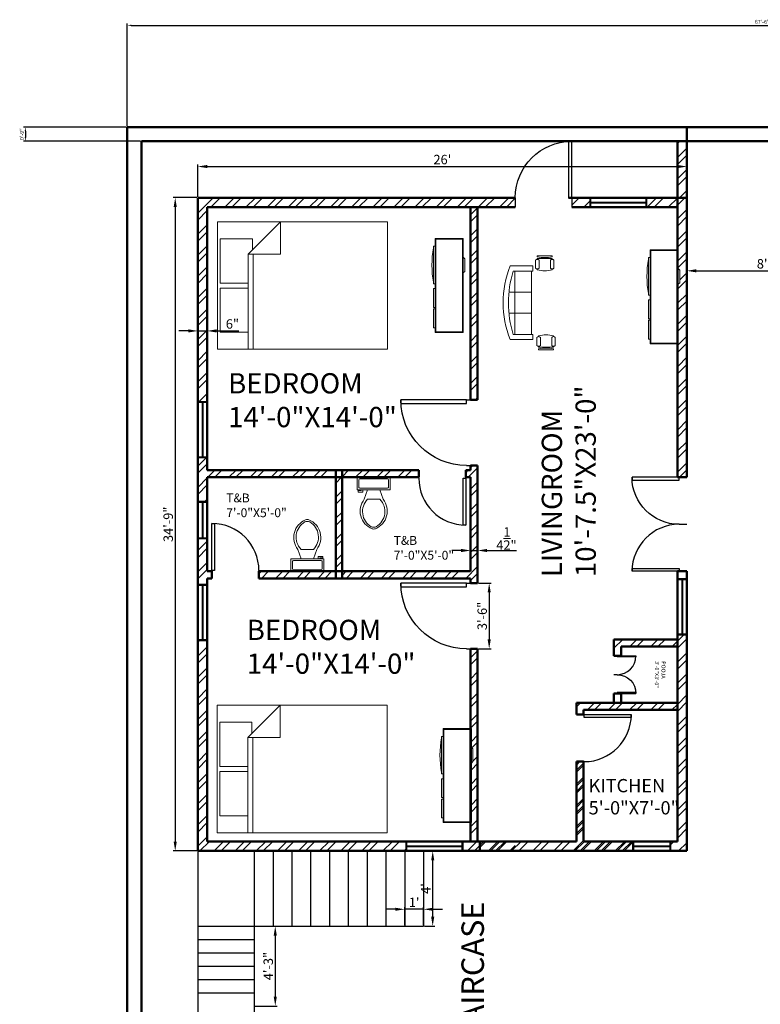
# Model space of a CAD drawing. Units: inches. Extents: x -12550 to 6516, y 1273 to 18700.
# Tile 10 of 19: x 3066 to 3538, y 1958 to 2587. Entities that reach past the tile are written whole.
import ezdxf

# ---------------------------------------------------------------- set-up
doc = ezdxf.new("R2010")
doc.units = ezdxf.units.IN
for name, color, linetype, lineweight in [('A-ANNO-DIMS', 2, 'Continuous', 18), ('A-AREA-IDEN', 1, 'Continuous', 18), ('A-DOOR', 5, 'Continuous', 25), ('A-FLOR-STRS', 6, 'Continuous', 25), ('A-FURN', 8, 'Continuous', 18), ('A-GLAZ', 3, 'Continuous', 25), ('A-WALL', 7, 'Continuous', 50), ('A-WALL-PATT', 8, 'Continuous', 13)]:
    doc.layers.add(name, color=color, linetype=linetype, lineweight=lineweight)
doc.styles.get("Standard").update_dxf_attribs({"font": 'arial.ttf'})
doc.dimstyles.new('ISO-25', dxfattribs={"dimtxt": 2.5, "dimasz": 2.5, "dimexe": 1.25, "dimexo": 0.625, "dimtad": 1, "dimlunit": 4, "dimtxsty": 'Standard', "dimcen": 2.5, "dimadec": 0, "dimazin": 0, "dimtfac": 1, "dimtmove": 0, "dimatfit": 3, "dimfxl": 1, "dimarcsym": 0})
pattern_1 = [(45, (1161.5385, 0), (-6.735192, 6.735192), []), (45, (1166.029, 0), (-6.735192, 6.735192), [])]
pattern_2 = [(45, (1161.5385, 567), (-6.735192, 6.735192), []), (45, (1166.029, 567), (-6.735192, 6.735192), [])]

# ---------------------------------------------------------------- blocks, each defined once
blk = doc.blocks.new('*U2')
for p, q in [((0, 0), (0, -5)), ((30, 0), (30, -5))]:
    blk.add_line(p, q)
blk.add_lwpolyline([(0, 0), (0, 30), (1.75, 30), (1.75, 0)], close=True)
blk.add_arc((0, 0), 30, 0, 90)
blk = doc.blocks.new('Bed - Queen')
for p, q in [((0, -80.00003), (0, 0)), ((0, 0), (59.99999, 0)), ((59.99999, 0), (59.99999, -80.00003)), ((7.99999, -1.2), (28.79998, -1.2)), ((7.99999, -14.4), (7.99999, -1.2)), ((28.79998, -1.2), (28.79998, -14.4)), ((31.19999, -1.2), (51.99999, -1.2)), ((31.19999, -14.4), (31.19999, -1.2)), ((51.99999, -1.2), (51.99999, -16.4)), ((0, -14.4), (44.8, -14.4)), ((44.8, -16.8), (0, -16.8)), ((59.99999, -29.6), (44.8, -14.4)), ((44.8, -14.4), (44.8, -29.6)), ((51.99999, -16.4), (46.79936, -16.4)), ((44.8, -29.6), (59.99999, -29.6)), ((59.99999, -80.00003), (0, -80.00003))]:
    blk.add_line(p, q)
blk = doc.blocks.new('Toilet - top')
for p, q in [((9.5, -6), (9.5, -2)), ((-10, -8.5), (-8, -8.5)), ((-10, -9.5), (-10, -8.5)), ((-7, -9.5), (-10, -9.5)), ((-8, -8.5), (-8, -8)), ((-7, -8), (-7, -9.5)), ((-4, -8), (-6, -14)), ((4, -8), (6, -14)), ((4, -14), (-4, -14))]:
    blk.add_line(p, q)
blk.add_lwpolyline([(10.5, -8), (10.5, 0), (-10.5, 0), (-10.5, -8)], close=True)
for points in [[(-9.5, -2), (-9.5, -6)], [(8.5, -1), (-8.5, -1)], [(-8.5, -7), (8.5, -7)]]:
    blk.add_lwpolyline(points)
for centre, radius, start, end in [((-8.62, -1.88), 0.884, 81.8699, 188.1301), ((-8.62, -6.12), 0.884, 171.8699, 278.1301), ((8.62, -1.88), 0.884, 351.8699, 98.1301), ((8.62, -6.12), 0.884, 261.8699, 8.1301), ((3.52, -21.58), 12.17, 141.46911, 247.97143), ((4.2, -21.82), 11.33, 136.36773, 238.94682), ((-3.52, -21.58), 12.17, 292.02843, 38.53071), ((-4.2, -21.82), 11.33, 301.05301, 43.63209), ((0, -27.88), 4, 245.73182, 294.26817), ((0, -29), 4, 254.86053, 285.13947)]:
    blk.add_arc(centre, radius, start, end)
blk = doc.blocks.new('Entertainment Center')
for p, q in [((-4, 0), (-5, -1)), ((4, 0), (-4, 0)), ((5, -1), (4, 0)), ((-17, -19), (-17, -1)), ((-17, -1), (43, -1)), ((-16.5, -18.5), (-16.5, -1.5)), ((-16.5, -1.5), (42.5, -1.5)), ((42.5, -1.5), (42.5, -18.5)), ((43, -1), (43, -19)), ((42.5, -18.5), (-16.5, -18.5)), ((43, -19), (-17, -19)), ((-12, -20), (-12, -19)), ((12, -20), (-12, -20)), ((12, -19), (12, -20)), ((15, -20), (15, -19)), ((27, -20), (15, -20)), ((27, -19), (27, -20)), ((28, -20), (28, -19)), ((40, -20), (28, -20)), ((40, -19), (40, -20))]:
    blk.add_line(p, q)
blk.add_arc((0, 40), 61, 259.6111, 280.3889)
blk = doc.blocks.new('Sofa - Roundback 7 ft.')
for p, q in [((-12.00002, -32.4421), (-12.00003, -6.5971)), ((11.99997, -32.4421), (11.99998, -6.5971)), ((-36.000027, -34), (-36.000027, -11.4696)), ((-35.999844, -13.3819), (35.9998, -13.3819)), ((35.99998, -34), (35.99998, -11.4696)), ((-36.000027, -32.4421), (35.99998, -32.4421))]:
    blk.add_line(p, q)
for points in [[(-36.000027, -34), (-42.000027, -34), (-42.000027, -8)], [(41.99998, -8), (41.99998, -34), (35.99998, -34)]]:
    blk.add_lwpolyline(points)
for centre, radius, start, end in [((0, -114.25), 114.25, 68.43141, 111.5686), ((-0.00001, -127.1968), 121.1968, 72.72033, 107.2797)]:
    blk.add_arc(centre, radius, start, end)
blk = doc.blocks.new('Chair - Desk')
for p, q in [((-8.5, 0), (-8.5, -1)), ((-8.5, 0), (8.5, 0)), ((8.5, 0), (8.5, -1)), ((-10.5, -5), (-10.5, -14)), ((-8.5, -3), (-8.5, -4)), ((-8.5, -3), (8.5, -3)), ((-6.5, -14), (-6.5, -5)), ((-2, -3), (-2, -1.9355)), ((2, -1.9576), (2, -3)), ((6.5, -5), (6.5, -14)), ((8.5, -3), (8.5, -4)), ((10.5, -14), (10.5, -5)), ((-8.5, -15), (-8.5, -16)), ((8.5, -15), (8.5, -16))]:
    blk.add_line(p, q)
for centre, radius, start, end in [((-8.5, -6.5), 2.5, 36.8699, 143.1301), ((0, 34.625), 36.625, 256.5803, 283.4197), ((8.5, -6.5), 2.5, 36.8699, 143.1301), ((-8.5, -12.5), 2.5, 216.8699, 323.1301), ((0, 19.625), 36.625, 256.5803, 283.4197), ((8.5, -12.5), 2.5, 216.8699, 323.1301)]:
    blk.add_arc(centre, radius, start, end)
blk = doc.blocks.new('*D25')
at = {"layer": 'A-ANNO-DIMS', "color": 0, "lineweight": -2, "transparency": 16777216}
for p, q in [((3179.23, 2388.03), (3179.23, 2389.43)), ((3185.23, 2388.03), (3185.23, 2389.43)), ((3173.23, 2388.18), (3167.23, 2388.18)), ((3179.23, 2388.18), (3185.23, 2388.18)), ((3191.23, 2388.18), (3205.41, 2388.18))]:
    blk.add_line(p, q, dxfattribs=at)
at = {"layer": 'A-ANNO-DIMS', "color": 0, "transparency": 16777216}
for points in [[(3173.23, 2389.18), (3173.23, 2387.18), (3179.23, 2388.18)], [(3191.23, 2389.18), (3191.23, 2387.18), (3185.23, 2388.18)]]:
    blk.add_solid(points, dxfattribs=at)
at = {"layer": 'Defpoints', "color": 0, "transparency": 16777216}
for p in [(3179.23, 2387.4), (3185.23, 2388.18), (3185.23, 2387.4)]:
    blk.add_point(p, dxfattribs=at)
at = {"layer": 'A-ANNO-DIMS', "color": 0, "transparency": 16777216, "insert": (3201.32, 2391.87), "char_height": 6, "attachment_point": 5}
blk.add_mtext('6"', dxfattribs=at)
blk = doc.blocks.new('*D26')
at = {"layer": 'A-ANNO-DIMS', "color": 0, "lineweight": -2, "transparency": 16777216}
for p, q in [((3353.23, 2251.78), (3353.23, 2246.78)), ((3357.73, 2251.78), (3357.73, 2246.78)), ((3347.23, 2248.03), (3341.23, 2248.03)), ((3353.23, 2248.03), (3357.73, 2248.03)), ((3363.73, 2248.03), (3382.49, 2248.03))]:
    blk.add_line(p, q, dxfattribs=at)
at = {"layer": 'A-ANNO-DIMS', "color": 0, "transparency": 16777216}
for points in [[(3347.23, 2249.03), (3347.23, 2247.03), (3353.23, 2248.03)], [(3363.73, 2249.03), (3363.73, 2247.03), (3357.73, 2248.03)]]:
    blk.add_solid(points, dxfattribs=at)
at = {"layer": 'Defpoints', "color": 0, "transparency": 16777216}
for p in [(3353.23, 2252.41), (3357.73, 2252.41), (3357.73, 2248.03)]:
    blk.add_point(p, dxfattribs=at)
at = {"layer": 'A-ANNO-DIMS', "color": 0, "transparency": 16777216, "insert": (3376.11, 2255.68), "char_height": 6, "attachment_point": 5}
blk.add_mtext('4{\\H1x;\\S1/2;}"', dxfattribs=at)
blk = doc.blocks.new('*D33')
at = {"layer": 'A-ANNO-DIMS', "color": 0, "lineweight": -2, "transparency": 16777216}
for p, q in [((3358.35, 2227.25), (3366.36, 2227.25)), ((3365.11, 2221.25), (3365.11, 2191.25)), ((3358.35, 2185.25), (3366.36, 2185.25))]:
    blk.add_line(p, q, dxfattribs=at)
at = {"layer": 'A-ANNO-DIMS', "color": 0, "transparency": 16777216}
for points in [[(3364.11, 2221.25), (3366.11, 2221.25), (3365.11, 2227.25)], [(3364.11, 2191.25), (3366.11, 2191.25), (3365.11, 2185.25)]]:
    blk.add_solid(points, dxfattribs=at)
at = {"layer": 'Defpoints', "color": 0, "transparency": 16777216}
for p in [(3357.73, 2227.25), (3357.73, 2185.25), (3365.11, 2185.25)]:
    blk.add_point(p, dxfattribs=at)
at = {"layer": 'A-ANNO-DIMS', "color": 0, "transparency": 16777216, "insert": (3361.42, 2206.25), "char_height": 6, "attachment_point": 5, "rotation": 90}
blk.add_mtext('3\'-6"', dxfattribs=at)
blk = doc.blocks.new('*D34')
at = {"layer": 'A-ANNO-DIMS', "color": 0, "lineweight": -2, "transparency": 16777216}
for p, q in [((3323.85, 2056.25), (3330.33, 2056.25)), ((3329.08, 2014.25), (3329.08, 2050.25)), ((3323.85, 2008.25), (3330.33, 2008.25))]:
    blk.add_line(p, q, dxfattribs=at)
at = {"layer": 'A-ANNO-DIMS', "color": 0, "transparency": 16777216}
for points in [[(3328.08, 2050.25), (3330.08, 2050.25), (3329.08, 2056.25)], [(3328.08, 2014.25), (3330.08, 2014.25), (3329.08, 2008.25)]]:
    blk.add_solid(points, dxfattribs=at)
at = {"layer": 'Defpoints', "color": 0, "transparency": 16777216}
for p in [(3323.23, 2056.25), (3329.08, 2056.25), (3323.23, 2008.25)]:
    blk.add_point(p, dxfattribs=at)
at = {"layer": 'A-ANNO-DIMS', "color": 0, "transparency": 16777216, "insert": (3325.46, 2032.25), "char_height": 6, "attachment_point": 5, "rotation": 90}
blk.add_mtext("4'", dxfattribs=at)
blk = doc.blocks.new('*D35')
at = {"layer": 'A-ANNO-DIMS', "color": 0, "lineweight": -2, "transparency": 16777216}
for p, q in [((3305.23, 2019.01), (3299.23, 2019.01)), ((3311.23, 2008.87), (3311.23, 2020.26)), ((3323.23, 2019.01), (3311.23, 2019.01)), ((3323.23, 2008.87), (3323.23, 2020.26)), ((3329.23, 2019.01), (3335.23, 2019.01))]:
    blk.add_line(p, q, dxfattribs=at)
at = {"layer": 'A-ANNO-DIMS', "color": 0, "transparency": 16777216}
for points in [[(3305.23, 2020.01), (3305.23, 2018.01), (3311.23, 2019.01)], [(3329.23, 2020.01), (3329.23, 2018.01), (3323.23, 2019.01)]]:
    blk.add_solid(points, dxfattribs=at)
at = {"layer": 'Defpoints', "color": 0, "transparency": 16777216}
for p in [(3311.23, 2019.01), (3311.23, 2008.25), (3323.23, 2008.25)]:
    blk.add_point(p, dxfattribs=at)
at = {"layer": 'A-ANNO-DIMS', "color": 0, "transparency": 16777216, "insert": (3317.23, 2022.65), "char_height": 6, "attachment_point": 5}
blk.add_mtext("1'", dxfattribs=at)
blk = doc.blocks.new('*D36')
at = {"layer": 'A-ANNO-DIMS', "color": 0, "lineweight": -2, "transparency": 16777216}
for p, q in [((3215.85, 2008.25), (3229.9, 2008.25)), ((3228.65, 2002.25), (3228.65, 1963.25)), ((3215.85, 1957.25), (3229.9, 1957.25))]:
    blk.add_line(p, q, dxfattribs=at)
at = {"layer": 'A-ANNO-DIMS', "color": 0, "transparency": 16777216}
for points in [[(3227.65, 2002.25), (3229.65, 2002.25), (3228.65, 2008.25)], [(3227.65, 1963.25), (3229.65, 1963.25), (3228.65, 1957.25)]]:
    blk.add_solid(points, dxfattribs=at)
at = {"layer": 'Defpoints', "color": 0, "transparency": 16777216}
for p in [(3215.23, 2008.25), (3215.23, 1957.25), (3228.65, 1957.25)]:
    blk.add_point(p, dxfattribs=at)
at = {"layer": 'A-ANNO-DIMS', "color": 0, "transparency": 16777216, "insert": (3224.96, 1982.75), "char_height": 6, "attachment_point": 5, "rotation": 90}
blk.add_mtext('4\'-3"', dxfattribs=at)
blk = doc.blocks.new('*D29')
at = {"layer": 'A-ANNO-DIMS', "color": 0, "lineweight": -2, "transparency": 16777216}
for p, q in [((3178.6, 2473.25), (3163.57, 2473.25)), ((3164.82, 2467.25), (3164.82, 2062.25)), ((3178.6, 2056.25), (3163.57, 2056.25))]:
    blk.add_line(p, q, dxfattribs=at)
at = {"layer": 'A-ANNO-DIMS', "color": 0, "transparency": 16777216}
for points in [[(3163.82, 2467.25), (3165.82, 2467.25), (3164.82, 2473.25)], [(3163.82, 2062.25), (3165.82, 2062.25), (3164.82, 2056.25)]]:
    blk.add_solid(points, dxfattribs=at)
at = {"layer": 'Defpoints', "color": 0, "transparency": 16777216}
for p in [(3179.23, 2473.25), (3164.82, 2056.25), (3179.23, 2056.25)]:
    blk.add_point(p, dxfattribs=at)
at = {"layer": 'A-ANNO-DIMS', "color": 0, "transparency": 16777216, "insert": (3161.13, 2264.75), "char_height": 6, "attachment_point": 5, "rotation": 90}
blk.add_mtext('34\'-9"', dxfattribs=at)
blk = doc.blocks.new('*D32')
at = {"layer": 'A-ANNO-DIMS', "color": 0, "lineweight": -2, "transparency": 16777216}
for p, q in [((3179.23, 2473.87), (3179.23, 2494.36)), ((3185.23, 2493.11), (3485.23, 2493.11)), ((3491.23, 2473.87), (3491.23, 2494.36))]:
    blk.add_line(p, q, dxfattribs=at)
at = {"layer": 'A-ANNO-DIMS', "color": 0, "transparency": 16777216}
for points in [[(3185.23, 2494.11), (3185.23, 2492.11), (3179.23, 2493.11)], [(3485.23, 2494.11), (3485.23, 2492.11), (3491.23, 2493.11)]]:
    blk.add_solid(points, dxfattribs=at)
at = {"layer": 'Defpoints', "color": 0, "transparency": 16777216}
for p in [(3491.23, 2493.11), (3179.23, 2473.25), (3491.23, 2473.25)]:
    blk.add_point(p, dxfattribs=at)
at = {"layer": 'A-ANNO-DIMS', "color": 0, "transparency": 16777216, "insert": (3335.23, 2496.8), "char_height": 6, "attachment_point": 5}
blk.add_mtext("26'", dxfattribs=at)
blk = doc.blocks.new('*D27')
at = {"layer": 'A-ANNO-DIMS', "color": 0, "lineweight": -2, "transparency": 16777216}
for p, q in [((3491.23, 2407.12), (3491.23, 2427.81)), ((3497.23, 2426.56), (3581.23, 2426.56)), ((3587.23, 2407.12), (3587.23, 2427.81))]:
    blk.add_line(p, q, dxfattribs=at)
at = {"layer": 'A-ANNO-DIMS', "color": 0, "transparency": 16777216}
for points in [[(3497.23, 2427.56), (3497.23, 2425.56), (3491.23, 2426.56)], [(3581.23, 2427.56), (3581.23, 2425.56), (3587.23, 2426.56)]]:
    blk.add_solid(points, dxfattribs=at)
at = {"layer": 'Defpoints', "color": 0, "transparency": 16777216}
for p in [(3587.23, 2426.56), (3491.23, 2406.5), (3587.23, 2406.5)]:
    blk.add_point(p, dxfattribs=at)
at = {"layer": 'A-ANNO-DIMS', "color": 0, "transparency": 16777216, "insert": (3539.23, 2430.25), "char_height": 6, "attachment_point": 5}
blk.add_mtext("8'", dxfattribs=at)
blk = doc.blocks.new('WIN-3FT')
for p, q in [((0, 0), (0, 6)), ((0, 6), (36.02, 6)), ((36.02, 0), (0, 0)), ((0.5, 0), (0.5, 6)), ((35.52, 3.2), (0.5, 3.2)), ((35.52, 2.8), (0.5, 2.8)), ((35.52, 6), (35.52, 0)), ((36.02, 6), (36.02, 0))]:
    blk.add_line(p, q)
blk = doc.blocks.new('WIN-2FT')
for p, q in [((0, 0), (0, 24.02)), ((0, 24.02), (6, 24.02)), ((0, 23.52), (6, 23.52)), ((2.8, 0.5), (2.8, 23.52)), ((3.2, 0.5), (3.2, 23.52)), ((6, 24.02), (6, 0)), ((6, 0.5), (0, 0.5)), ((6, 0), (0, 0))]:
    blk.add_line(p, q)
blk = doc.blocks.new('*D103')
at = {"layer": 'A-ANNO-DIMS', "color": 0, "lineweight": -2, "transparency": 16777216}
for p, q in [((3134.23, 2518.87), (3134.23, 2584.5)), ((3136.73, 2583.25), (3941.73, 2583.25)), ((3944.23, 2518.87), (3944.23, 2584.5))]:
    blk.add_line(p, q, dxfattribs=at)
at = {"layer": 'A-ANNO-DIMS', "color": 0, "transparency": 16777216}
for points in [[(3136.73, 2583.66), (3136.73, 2582.83), (3134.23, 2583.25)], [(3941.73, 2583.66), (3941.73, 2582.83), (3944.23, 2583.25)]]:
    blk.add_solid(points, dxfattribs=at)
at = {"layer": 'Defpoints', "color": 0, "transparency": 16777216}
for p in [(3944.23, 2583.25), (3134.23, 2518.25), (3944.23, 2518.25)]:
    blk.add_point(p, dxfattribs=at)
at = {"layer": 'A-ANNO-DIMS', "color": 0, "transparency": 16777216, "insert": (3539.23, 2585.15), "char_height": 2.5, "attachment_point": 5}
blk.add_mtext('67\'-6"', dxfattribs=at)
blk = doc.blocks.new('*D111')
at = {"layer": 'A-ANNO-DIMS', "color": 0, "lineweight": -2, "transparency": 16777216}
for p, q in [((3133.6, 2518.25), (3067.98, 2518.25)), ((3069.23, 2515.75), (3069.23, 2511.75)), ((3142.6, 2509.25), (3067.98, 2509.25))]:
    blk.add_line(p, q, dxfattribs=at)
at = {"layer": 'A-ANNO-DIMS', "color": 0, "transparency": 16777216}
for points in [[(3068.81, 2515.75), (3069.64, 2515.75), (3069.23, 2518.25)], [(3068.81, 2511.75), (3069.64, 2511.75), (3069.23, 2509.25)]]:
    blk.add_solid(points, dxfattribs=at)
at = {"layer": 'Defpoints', "color": 0, "transparency": 16777216}
for p in [(3134.23, 2518.25), (3069.23, 2509.25), (3143.23, 2509.25)]:
    blk.add_point(p, dxfattribs=at)
at = {"layer": 'A-ANNO-DIMS', "color": 0, "transparency": 16777216, "insert": (3067.33, 2513.75), "char_height": 2.5, "attachment_point": 5, "rotation": 90}
blk.add_mtext('0\'-9"', dxfattribs=at)

msp = doc.modelspace()

# ---------------------------------------------------------------- hatches: boundary and pattern name
at = {"layer": 'A-WALL-PATT'}
h = msp.add_hatch(dxfattribs=at)
h.set_pattern_fill('ANSI32', color=256)
h.set_pattern_definition(pattern_1)
h.paths.add_polyline_path([(3491.227, 2509.247), (3485.227, 2509.247), (3485.227, 2473.247), (3491.227, 2473.247)])
h = msp.add_hatch(dxfattribs=at)
h.set_pattern_fill('ANSI32', color=256)
h.set_pattern_definition(pattern_2)
h.paths.add_polyline_path([(3185.227, 2467.247), (3359.227, 2467.247), (3359.227, 2473.247), (3179.227, 2473.247), (3179.227, 2343.138), (3185.227, 2343.138)])
h = msp.add_hatch(dxfattribs=at)
h.set_pattern_fill('ANSI32', color=256)
h.set_pattern_definition(pattern_2)
h.paths.add_polyline_path([(3417.727, 2473.247), (3417.727, 2467.247), (3429.479, 2467.247), (3429.479, 2473.247)])
h.paths.add_polyline_path([(3381.727, 2467.247), (3381.727, 2473.247), (3359.227, 2473.247), (3359.227, 2467.247)])
h = msp.add_hatch(dxfattribs=at)
h.set_pattern_fill('ANSI32', color=256)
h.set_pattern_definition(pattern_2)
h.paths.add_polyline_path([(3491.227, 2473.247), (3465.496, 2473.247), (3465.496, 2467.247), (3485.227, 2467.247), (3485.227, 2439.972), (3485.727, 2439.972), (3485.727, 2427.972), (3486.727, 2426.972), (3486.727, 2418.972), (3485.727, 2417.972), (3485.727, 2379.972), (3485.227, 2294.747), (3486.227, 2294.747), (3491.227, 2294.747)])
h = msp.add_hatch(dxfattribs=at)
h.set_pattern_fill('ANSI32', color=256)
h.set_pattern_definition(pattern_2)
h.paths.add_polyline_path([(3357.727, 2467.247), (3353.227, 2467.247), (3353.227, 2344.247), (3357.727, 2344.247)], flags=17)
h = msp.add_hatch(dxfattribs=at)
h.set_pattern_fill('ANSI32', color=256)
h.set_pattern_definition(pattern_2)
h.paths.add_polyline_path([(3267.227, 2299.247), (3185.227, 2299.247), (3185.227, 2307.121), (3179.227, 2307.121), (3179.227, 2279.466), (3185.227, 2279.466), (3185.227, 2294.747), (3267.227, 2294.747)])
h = msp.add_hatch(dxfattribs=at)
h.set_pattern_fill('ANSI32', color=256)
h.set_pattern_definition(pattern_2)
h.paths.add_polyline_path([(3357.727, 2302.247), (3353.227, 2302.247), (3353.227, 2299.247), (3350.227, 2299.247), (3350.227, 2294.747), (3353.227, 2294.747), (3353.227, 2234.747), (3271.227, 2234.747), (3271.227, 2230.247), (3353.227, 2230.247), (3353.227, 2227.247), (3357.727, 2227.247)])
h = msp.add_hatch(dxfattribs=at)
h.set_pattern_fill('ANSI32', color=256)
h.set_pattern_definition(pattern_2)
h.paths.add_polyline_path([(3271.227, 2294.747), (3267.227, 2294.747), (3267.227, 2234.747), (3271.227, 2234.747)])
h = msp.add_hatch(dxfattribs=at)
h.set_pattern_fill('ANSI32', color=256)
h.set_pattern_definition(pattern_2)
h.paths.add_polyline_path([(3320.227, 2299.247), (3271.227, 2299.247), (3271.227, 2294.747), (3320.227, 2294.747)], flags=17)
h = msp.add_hatch(dxfattribs=at)
h.set_pattern_fill('ANSI32', color=256)
h.set_pattern_definition(pattern_2)
h.paths.add_polyline_path([(3185.227, 2255.449), (3179.227, 2255.449), (3179.227, 2226.453), (3185.227, 2226.453), (3185.227, 2230.247), (3188.227, 2230.247), (3188.227, 2234.747), (3185.227, 2234.747)])
h = msp.add_hatch(dxfattribs=at)
h.set_pattern_fill('ANSI32', color=256)
h.set_pattern_definition(pattern_2)
h.paths.add_polyline_path([(3267.227, 2234.747), (3218.227, 2234.747), (3218.227, 2230.247), (3267.227, 2230.247)])
h = msp.add_hatch(dxfattribs=at)
h.set_pattern_fill('ANSI32', color=256)
h.set_pattern_definition(pattern_2)
h.paths.add_polyline_path([(3491.227, 2194.032), (3485.227, 2194.032), (3485.227, 2062.247), (3480.833, 2062.247), (3480.833, 2056.247), (3491.227, 2056.247)])
h = msp.add_hatch(dxfattribs=at)
h.set_pattern_fill('ANSI32', color=256)
h.set_pattern_definition(pattern_2)
h.paths.add_polyline_path([(3185.227, 2190.435), (3179.227, 2190.435), (3179.227, 2056.247), (3312.178, 2056.247), (3312.178, 2062.247), (3185.227, 2062.247)])
h = msp.add_hatch(dxfattribs=at)
h.set_pattern_fill('ANSI32', color=256)
h.set_pattern_definition(pattern_2)
h.paths.add_polyline_path([(3485.227, 2191.247), (3444.727, 2191.247), (3444.727, 2180.747), (3446.727, 2180.747), (3449.227, 2180.747), (3449.227, 2186.747), (3485.227, 2186.747)])
h = msp.add_hatch(dxfattribs=at)
h.set_pattern_fill('ANSI32', color=256)
h.set_pattern_definition(pattern_2)
h.paths.add_polyline_path([(3357.727, 2185.247), (3353.227, 2185.247), (3353.227, 2134.365), (3353.727, 2134.365), (3353.727, 2122.365), (3354.727, 2121.365), (3354.727, 2113.365), (3353.727, 2112.365), (3353.727, 2074.365), (3353.227, 2062.247), (3357.727, 2062.247)])
h = msp.add_hatch(dxfattribs=at)
h.set_pattern_fill('ANSI32', color=256)
h.set_pattern_definition(pattern_2)
h.paths.add_polyline_path([(3485.227, 2150.747), (3420.727, 2150.747), (3420.727, 2143.247), (3425.227, 2143.247), (3425.227, 2146.247), (3485.227, 2146.247)])
h = msp.add_hatch(dxfattribs=at)
h.set_pattern_fill('ANSI32', color=256)
h.set_pattern_definition(pattern_1)
h.paths.add_polyline_path([(3456.815, 2062.247), (3425.227, 2062.247), (3425.227, 2113.247), (3420.727, 2113.247), (3420.727, 2062.247), (3417.727, 2062.247), (3359.227, 2062.247), (3359.227, 2056.247), (3417.727, 2056.247), (3456.815, 2056.247)])
h = msp.add_hatch(dxfattribs=at)
h.set_pattern_fill('ANSI32', color=256)
h.set_pattern_definition(pattern_2)
h.paths.add_polyline_path([(3425.227, 2062.247), (3425.227, 2113.247), (3420.727, 2113.247), (3420.727, 2062.247), (3417.727, 2062.247), (3417.727, 2056.247), (3456.815, 2056.247), (3456.815, 2062.247)])
h = msp.add_hatch(dxfattribs=at)
h.set_pattern_fill('ANSI32', color=256)
h.set_pattern_definition(pattern_2)
h.paths.add_polyline_path([(3348.196, 2062.247), (3348.196, 2056.247), (3381.727, 2056.247), (3381.727, 2062.247)])

# ---------------------------------------------------------------- linework, layer by layer
at = {"layer": 'A-FLOR-STRS'}
for p, q in [((3359.227, 2056.247), (3179.227, 2056.247)), ((3179.227, 2056.247), (3179.227, 1906.247)), ((3215.227, 2056.247), (3215.227, 1906.247)), ((3227.227, 2056.247), (3227.227, 2008.247)), ((3239.227, 2056.247), (3239.227, 2008.247)), ((3251.227, 2056.247), (3251.227, 2008.247)), ((3263.227, 2056.247), (3263.227, 2008.247)), ((3275.227, 2056.247), (3275.227, 2008.247)), ((3287.227, 2056.247), (3287.227, 2008.247)), ((3299.227, 2056.247), (3299.227, 2008.247)), ((3311.227, 2056.247), (3311.227, 2008.247)), ((3323.227, 2056.247), (3323.227, 2008.247)), ((3179.227, 2008.247), (3323.227, 2008.247)), ((3179.227, 2008.247), (3323.227, 2008.247)), ((3179.227, 1999.747), (3215.227, 1999.747)), ((3179.227, 1991.247), (3215.227, 1991.247)), ((3179.227, 1982.747), (3215.227, 1982.747)), ((3179.227, 1974.247), (3215.227, 1974.247)), ((3179.227, 1965.747), (3215.227, 1965.747))]:
    msp.add_line(p, q, dxfattribs=at)
at = {"layer": 'A-WALL'}
for p, q in [((3134.227, 1444.247), (3134.227, 2518.247)), ((3134.227, 2518.247), (3944.227, 2518.247)), ((3491.227, 2294.747), (3491.227, 2518.247)), ((3143.227, 1453.247), (3143.227, 2509.247)), ((3143.227, 2509.247), (3935.227, 2509.247)), ((3715.627, 2509.247), (3415.627, 2509.247)), ((3485.227, 2294.747), (3485.227, 2509.247)), ((3381.727, 2473.247), (3179.227, 2473.247)), ((3179.227, 2068.324), (3179.227, 2473.247)), ((3491.227, 2473.247), (3415.627, 2473.247)), ((3381.727, 2467.247), (3185.227, 2467.247)), ((3185.227, 2299.247), (3185.227, 2467.247)), ((3353.227, 2344.247), (3353.227, 2467.247)), ((3357.727, 2344.247), (3357.727, 2467.247)), ((3485.227, 2467.247), (3417.727, 2467.247)), ((3357.727, 2344.247), (3353.227, 2344.247)), ((3353.227, 2299.247), (3353.227, 2302.247)), ((3353.227, 2299.247), (3353.227, 2302.247)), ((3353.227, 2302.247), (3357.727, 2302.247)), ((3357.727, 2227.247), (3357.727, 2302.247)), ((3320.227, 2299.247), (3185.227, 2299.247)), ((3320.227, 2294.747), (3185.227, 2294.747)), ((3185.227, 2234.747), (3185.227, 2294.747)), ((3267.227, 2230.247), (3267.227, 2299.247)), ((3271.227, 2230.247), (3271.227, 2299.247)), ((3320.227, 2294.747), (3320.227, 2299.247)), ((3353.227, 2299.247), (3350.227, 2299.247)), ((3353.227, 2299.247), (3350.227, 2299.247)), ((3350.227, 2299.247), (3350.227, 2294.747)), ((3353.227, 2294.747), (3350.227, 2294.747)), ((3353.227, 2234.747), (3353.227, 2294.747)), ((3491.227, 2294.747), (3485.227, 2294.747)), ((3188.227, 2234.747), (3185.227, 2234.747)), ((3188.227, 2230.247), (3188.227, 2234.747)), ((3353.227, 2234.747), (3218.227, 2234.747)), ((3218.227, 2234.747), (3353.227, 2234.747)), ((3218.227, 2234.747), (3218.227, 2230.247)), ((3491.227, 2234.747), (3485.227, 2234.747)), ((3485.227, 2062.247), (3485.227, 2234.747)), ((3491.227, 2056.247), (3491.227, 2234.747)), ((3188.227, 2230.247), (3185.227, 2230.247)), ((3185.227, 2062.247), (3185.227, 2230.247)), ((3185.227, 2230.247), (3188.227, 2230.247)), ((3353.227, 2230.247), (3218.227, 2230.247)), ((3353.227, 2227.247), (3353.227, 2230.247)), ((3357.727, 2227.247), (3353.227, 2227.247)), ((3357.727, 2230.247), (3357.727, 2227.247)), ((3485.227, 2191.247), (3444.727, 2191.247)), ((3444.727, 2180.747), (3444.727, 2191.247)), ((3353.227, 2062.247), (3353.227, 2185.247)), ((3353.227, 2185.247), (3357.727, 2185.247)), ((3357.727, 2062.247), (3357.727, 2185.247)), ((3485.227, 2186.747), (3449.227, 2186.747)), ((3449.227, 2180.747), (3449.227, 2186.747)), ((3444.727, 2180.747), (3449.227, 2180.747)), ((3444.727, 2150.747), (3444.727, 2156.747)), ((3449.227, 2156.747), (3444.727, 2156.747)), ((3449.227, 2150.747), (3449.227, 2156.747)), ((3449.227, 2150.747), (3449.227, 2156.747)), ((3485.227, 2150.747), (3420.727, 2150.747)), ((3420.727, 2143.247), (3420.727, 2150.747)), ((3444.727, 2150.747), (3444.727, 2155.747)), ((3425.227, 2143.247), (3420.727, 2143.247)), ((3485.227, 2146.247), (3425.227, 2146.247)), ((3425.227, 2143.247), (3425.227, 2146.247)), ((3425.227, 2146.247), (3425.227, 2143.247)), ((3420.727, 2062.247), (3420.727, 2113.247)), ((3420.727, 2113.247), (3425.227, 2113.247)), ((3425.227, 2062.247), (3425.227, 2113.247)), ((3179.227, 2056.247), (3179.227, 2068.324)), ((3417.727, 2062.247), (3185.227, 2062.247)), ((3381.727, 2062.247), (3357.727, 2062.247)), ((3359.227, 2056.247), (3359.227, 2062.247)), ((3420.727, 2062.247), (3417.727, 2062.247)), ((3420.727, 2062.247), (3417.727, 2062.247)), ((3485.227, 2062.247), (3425.227, 2062.247)), ((3417.727, 2056.247), (3179.227, 2056.247)), ((3491.227, 2056.247), (3417.727, 2056.247))]:
    msp.add_line(p, q, dxfattribs=at)

# ---------------------------------------------------------------- block references
at = {"layer": 'A-DOOR', "xscale": -1.199999999999999, "yscale": 1.199999999999999, "zscale": 1.199999999999999}
msp.add_blockref('*U2', (3417.727, 2473.247), dxfattribs=at)
at = {"layer": 'A-DOOR'}
for p, xscale, yscale, zscale, rotation in [((3350.727, 2344.247), -1.4, 1.4, 1.4, 90), ((3350.727, 2227.247), -1.4, 1.4, 1.4, 90), ((3446.727, 2180.747), 0.399999999999997, 0.399999999999997, 0.399999999999997, 270), ((3446.727, 2156.747), -0.399999999999997, 0.399999999999997, 0.399999999999997, 270)]:
    msp.add_blockref('*U2', p, dxfattribs=dict(at, xscale=xscale, yscale=yscale, zscale=zscale, rotation=rotation))
for p, rotation in [((3350.227, 2294.247), 180), ((3486.227, 2234.747), 90), ((3425.727, 2143.247), 270)]:
    msp.add_blockref('*U2', p, dxfattribs=dict(at, rotation=rotation))
at = {"layer": 'A-DOOR', "xscale": -1, "rotation": 90}
msp.add_blockref('*U2', (3486.227, 2294.747), dxfattribs=at)
at = {"layer": 'A-DOOR'}
msp.add_blockref('*U2', (3188.227, 2235.247), dxfattribs=at)
at = {"layer": 'A-FURN'}
for name, p, xscale, yscale, zscale, rotation in [('Bed - Queen', (3191.878, 2376.493), 1.354827908062564, 1.354827908062564, 1.354827908062564, 90), ('Sofa - Roundback 7 ft.', (3373.986, 2406.138), 0.5595223685495907, 0.5595223685495907, 0.5595223685495907, 90), ('Chair - Desk', (3401.426, 2376.138), 0.5595223685495907, 0.5595223685495907, 0.5595223685495907, 180), ('Bed - Queen', (3191.576, 2067.915), 1.354827908062564, 1.354827908062564, 1.354827908062564, 90)]:
    msp.add_blockref(name, p, dxfattribs=dict(at, xscale=xscale, yscale=yscale, zscale=zscale, rotation=rotation))
for name, p, rotation in [('Entertainment Center', (3349.568, 2430.204), 270), ('Entertainment Center', (3486.727, 2422.972), 270), ('Toilet - top', (3249.075, 2234.747), 180), ('Entertainment Center', (3354.727, 2117.365), 270)]:
    msp.add_blockref(name, p, dxfattribs=dict(at, rotation=rotation))
at = {"layer": 'A-FURN', "xscale": 0.5595223685495907, "yscale": 0.5595223685495907, "zscale": 0.5595223685495907}
msp.add_blockref('Chair - Desk', (3400.572, 2436.122), dxfattribs=at)
at = {"layer": 'A-FURN'}
msp.add_blockref('Toilet - top', (3291.439, 2294.747), dxfattribs=at)
at = {"layer": 'A-GLAZ'}
for name, p, rotation in [('WIN-3FT', (3465.496, 2473.247), 180), ('WIN-3FT', (3185.228, 2307.121), 90.00000000000188), ('WIN-2FT', (3185.227, 2279.467), 180), ('WIN-3FT', (3185.228, 2190.436), 90.0000000000021), ('WIN-3FT', (3491.228, 2194.032), 89.99999999999908), ('WIN-3FT', (3348.195, 2062.247), 180), ('WIN-2FT', (3456.815, 2062.247), 269.999999999998)]:
    msp.add_blockref(name, p, dxfattribs=dict(at, rotation=rotation))

# ---------------------------------------------------------------- texts
at = {"layer": 'A-AREA-IDEN', "char_height": 12.93169, "attachment_point": 1}
for insert in [(3198.564, 2361.217), (3210.445, 2203.812)]:
    msp.add_mtext('BEDROOM\\P14\'-0"X14\'-0"', dxfattribs=dict(at, insert=insert))
at = {"layer": 'A-AREA-IDEN', "insert": (3398.633, 2231.034), "char_height": 12.93169, "attachment_point": 1, "rotation": 90}
msp.add_mtext('LIVINGROOM\\P10\'-7.5"X23\'-0"', dxfattribs=at)
at = {"layer": 'A-AREA-IDEN', "attachment_point": 1}
for s, width, gutter_width, insert, char_height in [('T&B\\P7\'-0"X5\'-0"', 4.19569, 28.328, (3197.403, 2284.416), 5.66556), ('T&B\\P7\'-0"X5\'-0"', 4.19569, 28.328, (3304.165, 2257.282), 5.66556), ('KITCHEN\\P5\'-0"X7\'-0"', 1.29487, 42.422, (3428.549, 2102.176), 8.48435)]:
    msp.add_mtext_dynamic_manual_height_columns(s, width=width, gutter_width=gutter_width, heights=[0], dxfattribs=dict(at, insert=insert, char_height=char_height))
for s, width, gutter_width, insert, char_height, rotation in [('POOJA\\P3\'-0"X3\'-0"', 0.78585, 12.5, (3477.604, 2177.304), 2.5, 269.183853), ('STAIRCASE', 2.19144, 71.795, (3347.404, 1922.837), 14.3589, 90)]:
    msp.add_mtext_dynamic_manual_height_columns(s, width=width, gutter_width=gutter_width, heights=[0], dxfattribs=dict(at, insert=insert, char_height=char_height, rotation=rotation))

# ---------------------------------------------------------------- dimensions: what is measured, and where the dimension line sits
at = {"layer": 'A-ANNO-DIMS'}
for base, p1, p2, override, picture, middle in [((3944.227, 2583.247), (3134.227, 2518.247), (3944.227, 2518.247), {"dimdec": 1, "dimlfac": 1, "dimrnd": 0, "dimzin": 1, "dimdsep": 46, "dimlunit": 4, "dimfrac": 2}, '*D103', (3539.227, 2585.149)), ((3491.227, 2493.114), (3179.227, 2473.247), (3491.227, 2473.247), {"dimtxt": 6, "dimasz": 6, "dimclrd": 0, "dimclre": 0, "dimclrt": 0}, '*D32', (3335.227, 2496.802)), ((3587.227, 2426.562), (3491.227, 2406.497), (3587.227, 2406.497), {"dimtxt": 6, "dimasz": 6, "dimclrd": 0, "dimclre": 0, "dimclrt": 0}, '*D27', (3539.227, 2430.25)), ((3185.227, 2388.182), (3179.227, 2387.405), (3185.227, 2387.405), {"dimtxt": 6, "dimasz": 6, "dimclrd": 0, "dimclre": 0, "dimclrt": 0}, '*D25', (3201.317, 2391.871)), ((3357.727, 2248.034), (3353.227, 2252.406), (3357.727, 2252.406), {"dimtxt": 6, "dimasz": 6, "dimclrd": 0, "dimclre": 0, "dimclrt": 0}, '*D26', (3376.109, 2255.683)), ((3311.227, 2019.012), (3323.227, 2008.247), (3311.227, 2008.247), {"dimtxt": 6, "dimasz": 6, "dimclrd": 0, "dimclre": 0, "dimclrt": 0}, '*D35', (3317.227, 2022.65))]:
    dim = msp.add_linear_dim(base=base, p1=p1, p2=p2, dimstyle='ISO-25', override=override, dxfattribs=at)
    dim.commit()
    dim.dimension.update_dxf_attribs({"geometry": picture, "text_midpoint": middle})
for base, p1, p2, override, picture, middle in [((3069.227, 2509.247), (3134.227, 2518.247), (3143.227, 2509.247), {"dimdec": 1, "dimlfac": 1, "dimrnd": 0, "dimzin": 1, "dimdsep": 46, "dimlunit": 4, "dimfrac": 2}, '*D111', (3067.326, 2513.747)), ((3164.819, 2056.247), (3179.227, 2473.247), (3179.227, 2056.247), {"dimtxt": 6, "dimasz": 6, "dimclrd": 0, "dimclre": 0, "dimclrt": 0}, '*D29', (3161.128, 2264.747)), ((3365.111, 2185.247), (3357.727, 2227.247), (3357.727, 2185.247), {"dimtxt": 6, "dimasz": 6, "dimclrd": 0, "dimclre": 0, "dimclrt": 0}, '*D33', (3361.42, 2206.247)), ((3329.08, 2056.247), (3323.227, 2008.247), (3323.227, 2056.247), {"dimtxt": 6, "dimasz": 6, "dimclrd": 0, "dimclre": 0, "dimclrt": 0}, '*D34', (3325.455, 2032.247)), ((3228.649, 1957.247), (3215.227, 2008.247), (3215.227, 1957.247), {"dimtxt": 6, "dimasz": 6, "dimclrd": 0, "dimclre": 0, "dimclrt": 0}, '*D36', (3224.959, 1982.747))]:
    dim = msp.add_linear_dim(base=base, p1=p1, p2=p2, angle=90, dimstyle='ISO-25', override=override, dxfattribs=at)
    dim.commit()
    dim.dimension.update_dxf_attribs({"geometry": picture, "text_midpoint": middle})

doc.saveas('drawing.dxf')
